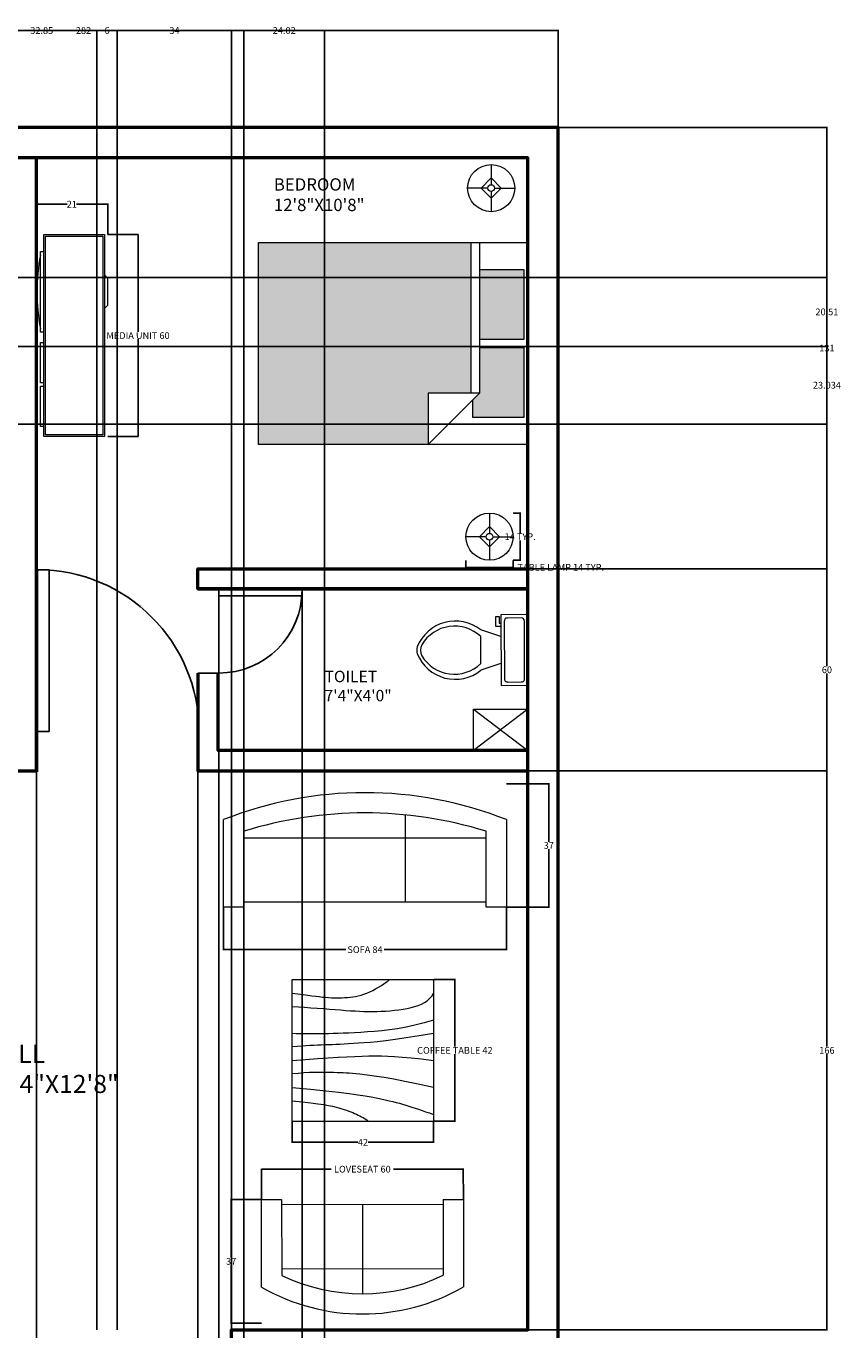
# Model space of a CAD drawing. Units: inches. Extents: x 32 to 429, y 30 to 648.
# Tile 3 of 3: x 187 to 429, y 261 to 648. Entities that reach past the tile are written whole.
import ezdxf

# ---------------------------------------------------------------- set-up
doc = ezdxf.new("R2010")
doc.units = ezdxf.units.IN
doc.header["$MEASUREMENT"] = 0
for name, color, linetype, lineweight in [('A-ANNO-DIMS', 2, 'Continuous', 18), ('A-AREA-IDEN', 7, 'Continuous', 25), ('A-DOOR', 4, 'Continuous', 25), ('A-FLOR-FIXT', 9, 'Continuous', 20), ('A-FURN', 9, 'Continuous', 18), ('A-FURN-PATT', 252, 'Continuous', 13), ('A-WALL', 7, 'Continuous', 50)]:
    doc.layers.add(name, color=color, linetype=linetype, lineweight=lineweight)
doc.styles.get("Standard").update_dxf_attribs({"font": 'arial.ttf'})
doc.dimstyles.get("Standard").update_dxf_attribs({"dimtxt": 2, "dimasz": 0.18, "dimexe": 0.18, "dimexo": 0.0625, "dimgap": 0.09, "dimtad": 0, "dimtih": 1, "dimtoh": 1, "dimrnd": 2, "dimzin": 0, "dimdsep": 46, "dimlunit": 3, "dimtxsty": 'Standard', "dimcen": 0.09, "dimadec": 0, "dimazin": 0, "dimtfac": 1, "dimtofl": 0, "dimtmove": 0, "dimatfit": 3, "dimfxl": 1, "dimtolj": 1, "dimtzin": 0, "dimarcsym": 0})

# ---------------------------------------------------------------- blocks, each defined once
blk = doc.blocks.new('*U3')
for p, q in [((9.5, -6), (9.5, -2)), ((-10, -8.5), (-8, -8.5)), ((-10, -9.5), (-10, -8.5)), ((-7, -9.5), (-10, -9.5)), ((-8, -8.5), (-8, -8)), ((-7, -8), (-7, -9.5)), ((-4, -8), (-6, -14)), ((4, -8), (6, -14)), ((4, -14), (-4, -14))]:
    blk.add_line(p, q)
blk.add_lwpolyline([(10.5, -8), (10.5, 0), (-10.5, 0), (-10.5, -8)], close=True)
for points in [[(-9.5, -2), (-9.5, -6)], [(8.5, -1), (-8.5, -1)], [(-8.5, -7), (8.5, -7)]]:
    blk.add_lwpolyline(points)
for centre, radius, start, end in [((-8.62, -1.88), 0.884, 81.8699, 188.1301), ((8.62, -1.88), 0.884, 351.8699, 98.1301), ((-8.62, -6.12), 0.884, 171.8699, 278.1301), ((8.62, -6.12), 0.884, 261.8699, 8.1301), ((3.52, -21.58), 12.17, 141.4691, 247.9714), ((4.2, -21.82), 11.33, 136.3677, 238.9468), ((-3.52, -21.58), 12.17, 292.0284, 38.5307), ((-4.2, -21.82), 11.33, 301.053, 43.6321), ((0, -27.88), 4, 245.7318, 294.2682), ((0, -29), 4, 254.8605, 285.1395)]:
    blk.add_arc(centre, radius, start, end)
blk = doc.blocks.new('*U6')
for p, q in [((-24, 0), (-24, 6)), ((0, 0), (0, 6))]:
    blk.add_line(p, q)
blk.add_lwpolyline([(0, 0), (0, -24), (-1.75, -24), (-1.75, 0)], close=True)
blk.add_arc((0, 0), 24, 180, 270)
blk = doc.blocks.new('*U8')
for p, q in [((-24, 0), (-24, 6)), ((0, 0), (0, 6))]:
    blk.add_line(p, q)
blk.add_lwpolyline([(0, 0), (0, -24), (-1.75, -24), (-1.75, 0)], close=True)
blk.add_arc((0, 0), 24, 180, 270)
blk = doc.blocks.new('Bed - Queen')
for p, q in [((0, -80.00003), (0, 0)), ((0, 0), (59.99999, 0)), ((59.99999, 0), (59.99999, -80.00003)), ((7.99999, -1.2), (28.79998, -1.2)), ((7.99999, -14.4), (7.99999, -1.2)), ((28.79998, -1.2), (28.79998, -14.4)), ((31.19999, -1.2), (51.99999, -1.2)), ((31.19999, -14.4), (31.19999, -1.2)), ((51.99999, -1.2), (51.99999, -16.4)), ((0, -14.4), (44.8, -14.4)), ((59.99999, -29.6), (44.8, -14.4)), ((44.8, -14.4), (44.8, -29.6)), ((44.8, -16.8), (0, -16.8)), ((51.99999, -16.4), (46.79936, -16.4)), ((44.8, -29.6), (59.99999, -29.6)), ((59.99999, -80.00003), (0, -80.00003))]:
    blk.add_line(p, q)
blk = doc.blocks.new('Entertainment Center')
for p, q in [((-4, 0), (-5, -1)), ((4, 0), (-4, 0)), ((5, -1), (4, 0)), ((-17, -19), (-17, -1)), ((-17, -1), (43, -1)), ((-16.5, -18.5), (-16.5, -1.5)), ((-16.5, -1.5), (42.5, -1.5)), ((42.5, -1.5), (42.5, -18.5)), ((43, -1), (43, -19)), ((43, -19), (-17, -19)), ((42.5, -18.5), (-16.5, -18.5)), ((-12, -20), (-12, -19)), ((12, -19), (12, -20)), ((15, -20), (15, -19)), ((27, -19), (27, -20)), ((28, -20), (28, -19)), ((40, -19), (40, -20)), ((12, -20), (-12, -20)), ((27, -20), (15, -20)), ((40, -20), (28, -20))]:
    blk.add_line(p, q)
blk.add_arc((0, 40), 61, 259.6111, 280.3889)
blk = doc.blocks.new('Lamp - Table')
for p, q in [((0, 7), (0, 1)), ((-1, 0), (-7, 0)), ((0, 3), (-3, 0)), ((-3, 0), (0, -3)), ((3, 0), (0, 3)), ((0, -3), (3, 0)), ((1, 0), (7, 0)), ((0, -1), (0, -7))]:
    blk.add_line(p, q)
for radius in [7, 1]:
    blk.add_circle((0, 0), radius)
blk = doc.blocks.new('Sofa - Roundback 7 ft.')
for p, q in [((-12.00002, -32.4421), (-12.00003, -6.5971)), ((11.99997, -32.4421), (11.99998, -6.5971)), ((-36.000027, -34), (-36.000027, -11.4696)), ((35.99998, -34), (35.99998, -11.4696)), ((-35.999844, -13.3819), (35.9998, -13.3819)), ((-36.000027, -32.4421), (35.99998, -32.4421))]:
    blk.add_line(p, q)
for points in [[(-36.000027, -34), (-42.000027, -34), (-42.000027, -8)], [(41.99998, -8), (41.99998, -34), (35.99998, -34)]]:
    blk.add_lwpolyline(points)
for centre, radius, start, end in [((0, -114.25), 114.25, 68.43141, 111.5686), ((-0.00001, -127.1968), 121.1968, 72.72033, 107.2797)]:
    blk.add_arc(centre, radius, start, end)
blk = doc.blocks.new('Sofa - Roundback Loveseat 5 ft.')
for p, q in [((0, -32.44198), (0, -5.99998)), ((-24, -33.99998), (-24, -11.46958)), ((24.00004, -33.99998), (24.00004, -11.46958)), ((-23.9998, -13.38178), (23.99986, -13.38178)), ((-24, -32.44198), (24.00004, -32.44198))]:
    blk.add_line(p, q)
for points in [[(-24, -33.99998), (-30, -33.99998), (-30, -7.99998)], [(30.00004, -7.99998), (30.00004, -33.99998), (24.00004, -33.99998)]]:
    blk.add_lwpolyline(points)
for centre, radius, start, end in [((0, -60.24998), 60.24998, 60.13715, 119.8628), ((0, -61.38438), 55.38444, 64.32083, 115.6792)]:
    blk.add_arc(centre, radius, start, end)
blk = doc.blocks.new('Table - Square Woodgrain 42 x 42 in.')
blk.add_line((0, -42), (42, -42))
for points in [[(0, -4), (1.704, -4.2172), (3.2358, -4.4188), (4.615, -4.604), (5.8615, -4.7721), (6.9951, -4.9224), (8.0357, -5.0541), (9.0031, -5.1667), (9.9171, -5.2594), (10.7951, -5.3316), (11.6445, -5.3836), (12.4702, -5.4157), (13.277, -5.4283), (14.0698, -5.4217), (14.8535, -5.3964), (15.6331, -5.3526), (16.4133, -5.2908), (17.1986, -5.2103), (17.9913, -5.1062), (18.793, -4.9727), (19.6056, -4.8038), (20.4307, -4.5937), (21.2701, -4.3365), (22.1256, -4.0262), (22.9989, -3.6571), (23.888, -3.2272), (24.7756, -2.7516), (25.6408, -2.2491), (26.4624, -1.7387), (27.2195, -1.2395), (27.891, -0.7703), (28.456, -0.3501), (28.8934, 0.002)], [(0, -42), (0, 0), (42, 0), (42, -42)], [(0, -8), (1.8203, -8.1001), (3.6741, -8.2149), (5.5411, -8.3408), (7.4011, -8.4741), (9.2339, -8.6112), (11.0193, -8.7484), (12.7371, -8.8821), (14.3671, -9.0086), (15.8954, -9.1246), (17.3337, -9.2278), (18.6997, -9.3159), (20.0116, -9.387), (21.2871, -9.4389), (22.5442, -9.4696), (23.8008, -9.477), (25.0749, -9.459), (26.3791, -9.4137), (27.7049, -9.3403), (29.0383, -9.2382), (30.3655, -9.1068), (31.6728, -8.9455), (32.9461, -8.7535), (34.1717, -8.5304), (35.3358, -8.2756), (36.4268, -7.9863), (37.443, -7.6521), (38.3849, -7.2603), (39.253, -6.7986), (40.048, -6.2542), (40.7705, -5.6147), (41.421, -4.8674), (42, -4)], [(42, -12), (39.1784, -12.8621), (36.4519, -13.5654), (33.8246, -14.1294), (31.3004, -14.5731), (28.8832, -14.9161), (26.577, -15.1775), (24.3858, -15.3768), (22.3136, -15.5332), (20.3622, -15.6632), (18.5254, -15.7718), (16.7947, -15.8612), (15.1618, -15.9338), (13.6183, -15.9916), (12.1558, -16.0369), (10.7659, -16.0718), (9.4403, -16.0987), (8.1703, -16.1191), (6.9461, -16.1325), (5.7577, -16.1377), (4.595, -16.1335), (3.4479, -16.1188), (2.3064, -16.0924), (1.1604, -16.0532), (0, -16)], [(42, -16), (37.6529, -16.7365), (33.8802, -17.329), (30.6179, -17.7961), (27.8015, -18.1561), (25.3668, -18.4275), (23.2497, -18.6288), (21.3859, -18.7785), (19.7111, -18.8949), (18.1693, -18.9939), (16.7375, -19.0795), (15.401, -19.1534), (14.1449, -19.217), (12.9544, -19.2717), (11.8148, -19.3191), (10.7113, -19.3606), (9.6291, -19.3976), (8.5534, -19.4323), (7.47, -19.4689), (6.3643, -19.5122), (5.222, -19.5672), (4.0288, -19.6386), (2.7703, -19.7313), (1.4321, -19.8501), (0, -20)], [(0, -24), (3.9243, -23.6805), (7.4766, -23.4138), (10.6891, -23.1954), (13.5943, -23.0205), (16.2247, -22.8847), (18.6125, -22.7832), (20.7903, -22.7116), (22.7903, -22.6651), (24.6563, -22.642), (26.4764, -22.6507), (28.35, -22.7024), (30.3766, -22.8084), (32.6555, -22.98), (35.2861, -23.2283), (38.3678, -23.5645), (42, -24)], [(42, -32), (37.392, -31.017), (33.4585, -30.2231), (30.1291, -29.5949), (27.3334, -29.109), (25.0009, -28.742), (23.0612, -28.4707), (21.4439, -28.2716), (20.0786, -28.1215), (18.8998, -28.0002), (17.8609, -27.9014), (16.9206, -27.8219), (16.0371, -27.7588), (15.1691, -27.709), (14.2748, -27.6693), (13.3128, -27.6368), (12.2415, -27.6083), (11.0295, -27.5824), (9.6867, -27.5643), (8.233, -27.5608), (6.6884, -27.5787), (5.0728, -27.6248), (3.4062, -27.7058), (1.7086, -27.8286), (0, -28)], [(0, -32), (5.4026, -32.5358), (9.9494, -33.019), (13.7424, -33.4553), (16.8834, -33.8505), (19.4743, -34.2106), (21.6171, -34.5413), (23.4136, -34.8486), (24.9657, -35.1382), (26.3614, -35.4156), (27.6332, -35.6841), (28.7995, -35.9467), (29.8788, -36.2064), (30.8897, -36.4661), (31.8507, -36.7288), (32.7802, -36.9973), (33.6968, -37.2747), (34.6175, -37.5635), (35.5531, -37.8651), (36.5128, -38.1805), (37.506, -38.5108), (38.5421, -38.8568), (39.6302, -39.2197), (40.7797, -39.6004), (42, -40)], [(0, -36), (3.0098, -36.2857), (5.5354, -36.5643), (7.6368, -36.8359), (9.374, -37.1009), (10.807, -37.3597), (11.9957, -37.6126), (13.0002, -37.8599), (13.8804, -38.102), (14.6874, -38.3393), (15.4365, -38.5729), (16.1338, -38.8041), (16.7858, -39.0341), (17.3987, -39.264), (17.9787, -39.4952), (18.5322, -39.7288), (19.0655, -39.9662), (19.5832, -40.2081), (20.0842, -40.4544), (20.5657, -40.7046), (21.0249, -40.9581), (21.459, -41.2144), (21.8653, -41.4731), (22.2409, -41.7335), (22.5831, -41.9951)]]:
    blk.add_lwpolyline(points)
blk = doc.blocks.new('*D19')
at = {"layer": 'A-ANNO-DIMS', "color": 0, "lineweight": -2, "transparency": 16777216}
for p, q in [((318, 489.44), (318, 487.22)), ((332, 489.44), (332, 487.22)), ((318.18, 487.4), (331.82, 487.4)), ((332, 487.4), (332.18, 487.4))]:
    blk.add_line(p, q, dxfattribs=at)
at = {"layer": 'A-ANNO-DIMS', "color": 0, "transparency": 16777216}
for points in [[(318.18, 487.43), (318.18, 487.37), (318, 487.4)], [(331.82, 487.43), (331.82, 487.37), (332, 487.4)]]:
    blk.add_solid(points, dxfattribs=at)
at = {"layer": 'Defpoints', "color": 0, "transparency": 16777216}
for p in [(318, 489.5), (332, 489.5), (332, 487.4)]:
    blk.add_point(p, dxfattribs=at)
at = {"layer": 'A-ANNO-DIMS', "color": 0, "transparency": 16777216, "insert": (346.17, 487.4), "char_height": 2, "attachment_point": 5}
blk.add_mtext('\\A1;TABLE LAMP 14 TYP.', dxfattribs=at)
blk = doc.blocks.new('*D20')
at = {"layer": 'A-ANNO-DIMS', "color": 0, "lineweight": -2, "transparency": 16777216}
for p, q in [((332.06, 503.5), (334.28, 503.5)), ((334.1, 503.32), (334.1, 497.59)), ((334.1, 489.68), (334.1, 495.41)), ((332.06, 489.5), (334.28, 489.5))]:
    blk.add_line(p, q, dxfattribs=at)
at = {"layer": 'A-ANNO-DIMS', "color": 0, "transparency": 16777216}
for points in [[(334.07, 503.32), (334.13, 503.32), (334.1, 503.5)], [(334.07, 489.68), (334.13, 489.68), (334.1, 489.5)]]:
    blk.add_solid(points, dxfattribs=at)
at = {"layer": 'Defpoints', "color": 0, "transparency": 16777216}
for p in [(332, 503.5), (334.1, 503.5), (332, 489.5)]:
    blk.add_point(p, dxfattribs=at)
at = {"layer": 'A-ANNO-DIMS', "color": 0, "transparency": 16777216, "insert": (334.1, 496.5), "char_height": 2, "attachment_point": 5}
blk.add_mtext('\\A1;14 TYP.', dxfattribs=at)
blk = doc.blocks.new('*D25')
at = {"layer": 'A-ANNO-DIMS', "color": 0, "lineweight": -2, "transparency": 16777216}
for p, q in [((211.65, 586.21), (220.76, 586.21)), ((220.58, 586.03), (220.58, 557.32)), ((220.58, 526.39), (220.58, 555.1)), ((211.65, 526.21), (220.76, 526.21))]:
    blk.add_line(p, q, dxfattribs=at)
at = {"layer": 'A-ANNO-DIMS', "color": 0, "transparency": 16777216}
for points in [[(220.55, 586.03), (220.61, 586.03), (220.58, 586.21)], [(220.55, 526.39), (220.61, 526.39), (220.58, 526.21)]]:
    blk.add_solid(points, dxfattribs=at)
at = {"layer": 'Defpoints', "color": 0, "transparency": 16777216}
for p in [(211.58, 586.21), (211.58, 526.21), (220.58, 526.21)]:
    blk.add_point(p, dxfattribs=at)
at = {"layer": 'A-ANNO-DIMS', "color": 0, "transparency": 16777216, "insert": (220.58, 556.21), "char_height": 2, "attachment_point": 5}
blk.add_mtext('\\A1;MEDIA UNIT 60', dxfattribs=at)
blk = doc.blocks.new('*D26')
at = {"layer": 'A-ANNO-DIMS', "color": 0, "lineweight": -2, "transparency": 16777216}
for p, q in [((190.25, 586.27), (190.25, 595.39)), ((190.43, 595.21), (199.57, 595.21)), ((211.4, 595.21), (202.26, 595.21)), ((211.58, 586.27), (211.58, 595.39))]:
    blk.add_line(p, q, dxfattribs=at)
at = {"layer": 'A-ANNO-DIMS', "color": 0, "transparency": 16777216}
for points in [[(190.43, 595.24), (190.43, 595.18), (190.25, 595.21)], [(211.4, 595.24), (211.4, 595.18), (211.58, 595.21)]]:
    blk.add_solid(points, dxfattribs=at)
at = {"layer": 'Defpoints', "color": 0, "transparency": 16777216}
for p in [(211.58, 595.21), (190.25, 586.21), (211.58, 586.21)]:
    blk.add_point(p, dxfattribs=at)
at = {"layer": 'A-ANNO-DIMS', "color": 0, "transparency": 16777216, "insert": (200.92, 595.21), "char_height": 2, "attachment_point": 5}
blk.add_mtext('\\A1;21', dxfattribs=at)
blk = doc.blocks.new('*D27')
at = {"layer": 'A-ANNO-DIMS', "color": 0, "lineweight": -2, "transparency": 16777216}
for p, q in [((246, 386.44), (246, 373.72)), ((330, 386.44), (330, 373.72)), ((246.18, 373.9), (282.29, 373.9)), ((329.82, 373.9), (293.71, 373.9))]:
    blk.add_line(p, q, dxfattribs=at)
at = {"layer": 'A-ANNO-DIMS', "color": 0, "transparency": 16777216}
for points in [[(246.18, 373.93), (246.18, 373.87), (246, 373.9)], [(329.82, 373.93), (329.82, 373.87), (330, 373.9)]]:
    blk.add_solid(points, dxfattribs=at)
at = {"layer": 'Defpoints', "color": 0, "transparency": 16777216}
for p in [(246, 386.5), (330, 386.5), (330, 373.9)]:
    blk.add_point(p, dxfattribs=at)
at = {"layer": 'A-ANNO-DIMS', "color": 0, "transparency": 16777216, "insert": (288, 373.9), "char_height": 2, "attachment_point": 5}
blk.add_mtext('\\A1;SOFA 84', dxfattribs=at)
blk = doc.blocks.new('*D28')
at = {"layer": 'A-ANNO-DIMS', "color": 0, "lineweight": -2, "transparency": 16777216}
for p, q in [((330.06, 423.17), (342.78, 423.17)), ((342.6, 422.99), (342.6, 405.95)), ((342.6, 386.68), (342.6, 403.72)), ((330.06, 386.5), (342.78, 386.5))]:
    blk.add_line(p, q, dxfattribs=at)
at = {"layer": 'A-ANNO-DIMS', "color": 0, "transparency": 16777216}
for points in [[(342.57, 422.99), (342.63, 422.99), (342.6, 423.17)], [(342.57, 386.68), (342.63, 386.68), (342.6, 386.5)]]:
    blk.add_solid(points, dxfattribs=at)
at = {"layer": 'Defpoints', "color": 0, "transparency": 16777216}
for p in [(330, 423.17), (342.6, 423.17), (330, 386.5)]:
    blk.add_point(p, dxfattribs=at)
at = {"layer": 'A-ANNO-DIMS', "color": 0, "transparency": 16777216, "insert": (342.6, 404.83), "char_height": 2, "attachment_point": 5}
blk.add_mtext('\\A1;37', dxfattribs=at)
blk = doc.blocks.new('*D29')
at = {"layer": 'A-ANNO-DIMS', "color": 0, "lineweight": -2, "transparency": 16777216}
for p, q in [((257.23, 299.74), (257.22, 308.86)), ((257.4, 308.68), (277.98, 308.71)), ((317.04, 308.76), (296.46, 308.74)), ((317.23, 299.83), (317.22, 308.94))]:
    blk.add_line(p, q, dxfattribs=at)
at = {"layer": 'A-ANNO-DIMS', "color": 0, "transparency": 16777216}
for points in [[(257.4, 308.71), (257.4, 308.65), (257.22, 308.68)], [(317.04, 308.79), (317.04, 308.73), (317.22, 308.76)]]:
    blk.add_solid(points, dxfattribs=at)
at = {"layer": 'Defpoints', "color": 0, "transparency": 16777216}
for p in [(257.22, 308.68), (257.23, 299.68), (317.23, 299.76)]:
    blk.add_point(p, dxfattribs=at)
at = {"layer": 'A-ANNO-DIMS', "color": 0, "transparency": 16777216, "insert": (287.22, 308.72), "char_height": 2, "attachment_point": 5}
blk.add_mtext('\\A1;LOVESEAT 60', dxfattribs=at)
blk = doc.blocks.new('*D30')
at = {"layer": 'A-ANNO-DIMS', "color": 0, "lineweight": -2, "transparency": 16777216}
for p, q in [((257.17, 299.68), (248.05, 299.67)), ((248.23, 299.49), (248.26, 282.45)), ((248.28, 263.18), (248.26, 280.22)), ((257.22, 263.01), (248.1, 263))]:
    blk.add_line(p, q, dxfattribs=at)
at = {"layer": 'A-ANNO-DIMS', "color": 0, "transparency": 16777216}
for points in [[(248.26, 299.49), (248.2, 299.49), (248.23, 299.67)], [(248.31, 263.18), (248.25, 263.18), (248.28, 263)]]:
    blk.add_solid(points, dxfattribs=at)
at = {"layer": 'Defpoints', "color": 0, "transparency": 16777216}
for p in [(257.23, 299.68), (248.28, 263), (257.28, 263.01)]:
    blk.add_point(p, dxfattribs=at)
at = {"layer": 'A-ANNO-DIMS', "color": 0, "transparency": 16777216, "insert": (248.26, 281.34), "char_height": 2, "attachment_point": 5}
blk.add_mtext('\\A1;37', dxfattribs=at)
blk = doc.blocks.new('*D31')
at = {"layer": 'A-ANNO-DIMS', "color": 0, "lineweight": -2, "transparency": 16777216}
for p, q in [((308.46, 365), (314.88, 365)), ((314.7, 364.82), (314.7, 345.13)), ((314.7, 323.18), (314.7, 342.88)), ((308.46, 323), (314.88, 323))]:
    blk.add_line(p, q, dxfattribs=at)
at = {"layer": 'A-ANNO-DIMS', "color": 0, "transparency": 16777216}
for points in [[(314.67, 364.82), (314.73, 364.82), (314.7, 365)], [(314.67, 323.18), (314.73, 323.18), (314.7, 323)]]:
    blk.add_solid(points, dxfattribs=at)
at = {"layer": 'Defpoints', "color": 0, "transparency": 16777216}
for p in [(308.4, 365), (314.7, 365), (308.4, 323)]:
    blk.add_point(p, dxfattribs=at)
at = {"layer": 'A-ANNO-DIMS', "color": 0, "transparency": 16777216, "insert": (314.7, 344), "char_height": 2, "attachment_point": 5}
blk.add_mtext('\\A1;COFFEE TABLE 42', dxfattribs=at)
blk = doc.blocks.new('*D32')
at = {"layer": 'A-ANNO-DIMS', "color": 0, "lineweight": -2, "transparency": 16777216}
for p, q in [((266.4, 322.94), (266.4, 316.52)), ((308.4, 322.94), (308.4, 316.52)), ((266.58, 316.7), (285.85, 316.7)), ((308.22, 316.7), (288.95, 316.7))]:
    blk.add_line(p, q, dxfattribs=at)
at = {"layer": 'A-ANNO-DIMS', "color": 0, "transparency": 16777216}
for points in [[(266.58, 316.73), (266.58, 316.67), (266.4, 316.7)], [(308.22, 316.73), (308.22, 316.67), (308.4, 316.7)]]:
    blk.add_solid(points, dxfattribs=at)
at = {"layer": 'Defpoints', "color": 0, "transparency": 16777216}
for p in [(266.4, 323), (308.4, 323), (308.4, 316.7)]:
    blk.add_point(p, dxfattribs=at)
at = {"layer": 'A-ANNO-DIMS', "color": 0, "transparency": 16777216, "insert": (287.4, 316.7), "char_height": 2, "attachment_point": 5}
blk.add_mtext('\\A1;42', dxfattribs=at)
blk = doc.blocks.new('*D33')
at = {"layer": 'A-ANNO-DIMS', "color": 0, "lineweight": -2, "transparency": 16777216}
for p, q in [((63.39, 618.06), (63.39, 646.97)), ((63.57, 646.79), (202.09, 646.79)), ((345.21, 646.79), (206.7, 646.79)), ((345.39, 618.06), (345.39, 646.97))]:
    blk.add_line(p, q, dxfattribs=at)
at = {"layer": 'A-ANNO-DIMS', "color": 0, "transparency": 16777216}
for points in [[(63.57, 646.82), (63.57, 646.76), (63.39, 646.79)], [(345.21, 646.82), (345.21, 646.76), (345.39, 646.79)]]:
    blk.add_solid(points, dxfattribs=at)
at = {"layer": 'Defpoints', "color": 0, "transparency": 16777216}
for p in [(345.39, 646.79), (63.39, 617.99), (345.39, 617.99)]:
    blk.add_point(p, dxfattribs=at)
at = {"layer": 'A-ANNO-DIMS', "color": 0, "transparency": 16777216, "insert": (204.39, 646.79), "char_height": 2, "attachment_point": 5}
blk.add_mtext('\\A1;282', dxfattribs=at)
blk = doc.blocks.new('*D40')
at = {"layer": 'A-ANNO-DIMS', "color": 0, "lineweight": -2, "transparency": 16777216}
for p, q in [((336.46, 426.99), (425.41, 426.99)), ((425.23, 426.81), (425.23, 345.1)), ((425.23, 261.17), (425.23, 342.88)), ((336.46, 260.99), (425.41, 260.99))]:
    blk.add_line(p, q, dxfattribs=at)
at = {"layer": 'A-ANNO-DIMS', "color": 0, "transparency": 16777216}
for points in [[(425.2, 426.81), (425.26, 426.81), (425.23, 426.99)], [(425.2, 261.17), (425.26, 261.17), (425.23, 260.99)]]:
    blk.add_solid(points, dxfattribs=at)
at = {"layer": 'Defpoints', "color": 0, "transparency": 16777216}
for p in [(336.39, 426.99), (425.23, 426.99), (336.39, 260.99)]:
    blk.add_point(p, dxfattribs=at)
at = {"layer": 'A-ANNO-DIMS', "color": 0, "transparency": 16777216, "insert": (425.23, 343.99), "char_height": 2, "attachment_point": 5}
blk.add_mtext('\\A1;166', dxfattribs=at)
blk = doc.blocks.new('*D41')
at = {"layer": 'A-ANNO-DIMS', "color": 0, "lineweight": -2, "transparency": 16777216}
for p, q in [((336.46, 486.99), (425.41, 486.99)), ((425.23, 486.81), (425.23, 458.1)), ((425.23, 427.17), (425.23, 455.88)), ((336.46, 426.99), (425.41, 426.99))]:
    blk.add_line(p, q, dxfattribs=at)
at = {"layer": 'A-ANNO-DIMS', "color": 0, "transparency": 16777216}
for points in [[(425.2, 486.81), (425.26, 486.81), (425.23, 486.99)], [(425.2, 427.17), (425.26, 427.17), (425.23, 426.99)]]:
    blk.add_solid(points, dxfattribs=at)
at = {"layer": 'Defpoints', "color": 0, "transparency": 16777216}
for p in [(336.39, 486.99), (425.23, 486.99), (336.39, 426.99)]:
    blk.add_point(p, dxfattribs=at)
at = {"layer": 'A-ANNO-DIMS', "color": 0, "transparency": 16777216, "insert": (425.23, 456.99), "char_height": 2, "attachment_point": 5}
blk.add_mtext('\\A1;60', dxfattribs=at)
blk = doc.blocks.new('*D42')
at = {"layer": 'A-ANNO-DIMS', "color": 0, "lineweight": -2, "transparency": 16777216}
for p, q in [((345.46, 617.99), (425.41, 617.99)), ((425.23, 617.81), (425.23, 553.6)), ((425.23, 487.17), (425.23, 551.38)), ((336.46, 486.99), (425.41, 486.99))]:
    blk.add_line(p, q, dxfattribs=at)
at = {"layer": 'A-ANNO-DIMS', "color": 0, "transparency": 16777216}
for points in [[(425.2, 617.81), (425.26, 617.81), (425.23, 617.99)], [(425.2, 487.17), (425.26, 487.17), (425.23, 486.99)]]:
    blk.add_solid(points, dxfattribs=at)
at = {"layer": 'Defpoints', "color": 0, "transparency": 16777216}
for p in [(345.39, 617.99), (425.23, 617.99), (336.39, 486.99)]:
    blk.add_point(p, dxfattribs=at)
at = {"layer": 'A-ANNO-DIMS', "color": 0, "transparency": 16777216, "insert": (425.23, 552.49), "char_height": 2, "attachment_point": 5}
blk.add_mtext('\\A1;131', dxfattribs=at)
blk = doc.blocks.new('*D45')
at = {"layer": 'A-ANNO-DIMS', "color": 0, "lineweight": -2, "transparency": 16777216}
for p, q in [((190.39, 426.93), (190.39, 31.01)), ((238.39, 426.93), (238.39, 31.01)), ((190.57, 31.19), (212.83, 31.19)), ((238.21, 31.19), (215.96, 31.19))]:
    blk.add_line(p, q, dxfattribs=at)
at = {"layer": 'A-ANNO-DIMS', "color": 0, "transparency": 16777216}
for points in [[(190.57, 31.22), (190.57, 31.16), (190.39, 31.19)], [(238.21, 31.22), (238.21, 31.16), (238.39, 31.19)]]:
    blk.add_solid(points, dxfattribs=at)
at = {"layer": 'Defpoints', "color": 0, "transparency": 16777216}
for p in [(190.39, 426.99), (238.39, 426.99), (238.39, 31.19)]:
    blk.add_point(p, dxfattribs=at)
at = {"layer": 'A-ANNO-DIMS', "color": 0, "transparency": 16777216, "insert": (214.39, 31.19), "char_height": 2, "attachment_point": 5}
blk.add_mtext('\\A1;48', dxfattribs=at)
blk = doc.blocks.new('*D46')
at = {"layer": 'A-ANNO-DIMS', "color": 0, "lineweight": -2, "transparency": 16777216}
for p, q in [((175.55, 261.06), (175.55, 646.97)), ((175.73, 646.79), (188.5, 646.79)), ((208.21, 646.79), (195.44, 646.79)), ((208.39, 261.06), (208.39, 646.97))]:
    blk.add_line(p, q, dxfattribs=at)
at = {"layer": 'A-ANNO-DIMS', "color": 0, "transparency": 16777216}
for points in [[(175.73, 646.82), (175.73, 646.76), (175.55, 646.79)], [(208.21, 646.82), (208.21, 646.76), (208.39, 646.79)]]:
    blk.add_solid(points, dxfattribs=at)
at = {"layer": 'Defpoints', "color": 0, "transparency": 16777216}
for p in [(208.39, 646.79), (175.55, 260.99), (208.39, 260.99)]:
    blk.add_point(p, dxfattribs=at)
at = {"layer": 'A-ANNO-DIMS', "color": 0, "transparency": 16777216, "insert": (191.97, 646.79), "char_height": 2, "attachment_point": 5}
blk.add_mtext('\\A1;32.85', dxfattribs=at)
blk = doc.blocks.new('*D47')
at = {"layer": 'A-ANNO-DIMS', "color": 0, "lineweight": -2, "transparency": 16777216}
for p, q in [((214.39, 261.06), (214.39, 646.97)), ((214.57, 646.79), (229.88, 646.79)), ((248.21, 646.79), (232.91, 646.79)), ((248.39, 261.06), (248.39, 646.97))]:
    blk.add_line(p, q, dxfattribs=at)
at = {"layer": 'A-ANNO-DIMS', "color": 0, "transparency": 16777216}
for points in [[(214.57, 646.82), (214.57, 646.76), (214.39, 646.79)], [(248.21, 646.82), (248.21, 646.76), (248.39, 646.79)]]:
    blk.add_solid(points, dxfattribs=at)
at = {"layer": 'Defpoints', "color": 0, "transparency": 16777216}
for p in [(248.39, 646.79), (214.39, 260.99), (248.39, 260.99)]:
    blk.add_point(p, dxfattribs=at)
at = {"layer": 'A-ANNO-DIMS', "color": 0, "transparency": 16777216, "insert": (231.39, 646.79), "char_height": 2, "attachment_point": 5}
blk.add_mtext('\\A1;34', dxfattribs=at)
blk = doc.blocks.new('*D48')
at = {"layer": 'A-ANNO-DIMS', "color": 0, "lineweight": -2, "transparency": 16777216}
for p, q in [((208.39, 261.06), (208.39, 646.97)), ((208.57, 646.79), (210.64, 646.79)), ((214.21, 646.79), (212.14, 646.79)), ((214.39, 261.06), (214.39, 646.97))]:
    blk.add_line(p, q, dxfattribs=at)
at = {"layer": 'A-ANNO-DIMS', "color": 0, "transparency": 16777216}
for points in [[(208.57, 646.82), (208.57, 646.76), (208.39, 646.79)], [(214.21, 646.82), (214.21, 646.76), (214.39, 646.79)]]:
    blk.add_solid(points, dxfattribs=at)
at = {"layer": 'Defpoints', "color": 0, "transparency": 16777216}
for p in [(214.39, 646.79), (208.39, 260.99), (214.39, 260.99)]:
    blk.add_point(p, dxfattribs=at)
at = {"layer": 'A-ANNO-DIMS', "color": 0, "transparency": 16777216, "insert": (211.39, 646.79), "char_height": 2, "attachment_point": 5}
blk.add_mtext('\\A1;6', dxfattribs=at)
blk = doc.blocks.new('*D50')
at = {"layer": 'A-ANNO-DIMS', "color": 0, "lineweight": -2, "transparency": 16777216}
for p, q in [((147.08, 552.99), (425.41, 552.99)), ((425.23, 552.81), (425.23, 542.59)), ((425.23, 530.14), (425.23, 540.36)), ((147.08, 529.96), (425.41, 529.96))]:
    blk.add_line(p, q, dxfattribs=at)
at = {"layer": 'A-ANNO-DIMS', "color": 0, "transparency": 16777216}
for points in [[(425.2, 552.81), (425.26, 552.81), (425.23, 552.99)], [(425.2, 530.14), (425.26, 530.14), (425.23, 529.96)]]:
    blk.add_solid(points, dxfattribs=at)
at = {"layer": 'Defpoints', "color": 0, "transparency": 16777216}
for p in [(147.02, 552.99), (147.02, 529.96), (425.23, 529.96)]:
    blk.add_point(p, dxfattribs=at)
at = {"layer": 'A-ANNO-DIMS', "color": 0, "transparency": 16777216, "insert": (425.23, 541.48), "char_height": 2, "attachment_point": 5}
blk.add_mtext('\\A1;23.034', dxfattribs=at)
blk = doc.blocks.new('*D51')
at = {"layer": 'A-ANNO-DIMS', "color": 0, "lineweight": -2, "transparency": 16777216}
for p, q in [((244.58, 478.88), (244.58, 31.01)), ((269.32, 478.88), (269.32, 31.01)), ((244.76, 31.19), (253.47, 31.19)), ((269.14, 31.19), (260.43, 31.19))]:
    blk.add_line(p, q, dxfattribs=at)
at = {"layer": 'A-ANNO-DIMS', "color": 0, "transparency": 16777216}
for points in [[(244.76, 31.22), (244.76, 31.16), (244.58, 31.19)], [(269.14, 31.22), (269.14, 31.16), (269.32, 31.19)]]:
    blk.add_solid(points, dxfattribs=at)
at = {"layer": 'Defpoints', "color": 0, "transparency": 16777216}
for p in [(244.58, 478.95), (269.32, 478.95), (269.32, 31.19)]:
    blk.add_point(p, dxfattribs=at)
at = {"layer": 'A-ANNO-DIMS', "color": 0, "transparency": 16777216, "insert": (256.95, 31.19), "char_height": 2, "attachment_point": 5}
blk.add_mtext('\\A1;24.74', dxfattribs=at)
blk = doc.blocks.new('*D52')
at = {"layer": 'A-ANNO-DIMS', "color": 0, "lineweight": -2, "transparency": 16777216}
for p, q in [((252, 232.11), (252, 646.97)), ((252.18, 646.79), (260.54, 646.79)), ((275.84, 646.79), (267.48, 646.79)), ((276.02, 232.11), (276.02, 646.97))]:
    blk.add_line(p, q, dxfattribs=at)
at = {"layer": 'A-ANNO-DIMS', "color": 0, "transparency": 16777216}
for points in [[(252.18, 646.82), (252.18, 646.76), (252, 646.79)], [(275.84, 646.82), (275.84, 646.76), (276.02, 646.79)]]:
    blk.add_solid(points, dxfattribs=at)
at = {"layer": 'Defpoints', "color": 0, "transparency": 16777216}
for p in [(276.02, 646.79), (252, 232.04), (276.02, 232.04)]:
    blk.add_point(p, dxfattribs=at)
at = {"layer": 'A-ANNO-DIMS', "color": 0, "transparency": 16777216, "insert": (264.01, 646.79), "char_height": 2, "attachment_point": 5}
blk.add_mtext('\\A1;24.02', dxfattribs=at)
blk = doc.blocks.new('*D56')
at = {"layer": 'A-ANNO-DIMS', "color": 0, "lineweight": -2, "transparency": 16777216}
for p, q in [((72.46, 573.5), (425.41, 573.5)), ((425.23, 573.32), (425.23, 564.36)), ((425.23, 553.17), (425.23, 562.14)), ((72.46, 552.99), (425.41, 552.99))]:
    blk.add_line(p, q, dxfattribs=at)
at = {"layer": 'A-ANNO-DIMS', "color": 0, "transparency": 16777216}
for points in [[(425.2, 573.32), (425.26, 573.32), (425.23, 573.5)], [(425.2, 553.17), (425.26, 553.17), (425.23, 552.99)]]:
    blk.add_solid(points, dxfattribs=at)
at = {"layer": 'Defpoints', "color": 0, "transparency": 16777216}
for p in [(72.39, 573.5), (425.23, 573.5), (72.39, 552.99)]:
    blk.add_point(p, dxfattribs=at)
at = {"layer": 'A-ANNO-DIMS', "color": 0, "transparency": 16777216, "insert": (425.23, 563.25), "char_height": 2, "attachment_point": 5}
blk.add_mtext('\\A1;20.51', dxfattribs=at)

msp = doc.modelspace()

# ---------------------------------------------------------------- hatches: boundary and pattern name
at = {"layer": 'A-FURN-PATT'}
h = msp.add_hatch(dxfattribs=at)
h.set_pattern_fill('DOTS', color=256)
h.paths.add_polyline_path([(335.194, 575.8763), (321.994, 575.8763), (321.994, 555.0763), (335.194, 555.0763)])
h.paths.add_polyline_path([(335.194, 552.6763), (321.994, 552.6763), (321.994, 539.0763), (319.994, 537.0763), (319.994, 531.8763), (335.194, 531.8763)])
h.paths.add_polyline_path([(319.594, 583.8763), (256.3939, 583.8763), (256.3939, 523.8763), (306.794, 523.8763), (306.794, 539.0763), (319.594, 539.0763)])
h = msp.add_hatch(dxfattribs=at)
h.set_pattern_fill('DOTS', color=256)
h.paths.add_polyline_path([(319.594, 583.8763), (256.3939, 583.8763), (256.3939, 523.8763), (306.794, 523.8763), (306.794, 539.0763), (319.594, 539.0763)])

# ---------------------------------------------------------------- linework, layer by layer
at = {"layer": 'A-FLOR-FIXT'}
for p, q in [((320.2761, 445.3289), (336.3942, 432.9929)), ((336.3942, 445.3289), (320.2761, 432.9929))]:
    msp.add_line(p, q, dxfattribs=at)
msp.add_lwpolyline([(336.3942, 432.9929), (320.2761, 432.9929), (320.2761, 445.3289), (336.3942, 445.3289)], close=True, dxfattribs=at)
at = {"layer": 'A-WALL'}
for points in [[(208.3942, 59.9929), (345.3942, 59.9929), (345.3942, 617.9929), (63.3942, 617.9929), (63.3942, 59.9929)], [(248.394, 254.9928), (248.394, 260.9928), (336.394, 260.9928), (336.394, 608.9928), (72.394, 608.9928), (72.394, 59.9928)], [(336.3942, 608.9929), (184.3942, 608.9929), (184.3942, 432.9929), (184.3942, 426.9929), (190.3942, 426.9929), (190.3942, 608.9929)], [(244.3942, 480.9929), (336.3942, 480.9929), (238.3942, 480.9929), (238.3942, 486.9929), (336.3942, 486.9929)], [(238.3942, 456.0096), (238.3942, 426.9929), (336.3942, 426.9929)], [(336.3942, 432.9929), (244.3942, 432.9929), (244.3942, 456.0073)]]:
    msp.add_lwpolyline(points, dxfattribs=at)

# ---------------------------------------------------------------- block references
at = {"layer": 'A-DOOR'}
for name, p, xscale, yscale, zscale, rotation in [('*U8', (190.681, 438.7075), 2.000008218349355, 2.000008218349355, 2.000008218349355, 180), ('*U6', (244.5793, 480.7509), 1.030886389251549, 1.030886389251549, 1.030886389251549, 90.00000000000003)]:
    msp.add_blockref(name, p, dxfattribs=dict(at, xscale=xscale, yscale=yscale, zscale=zscale, rotation=rotation))
at = {"layer": 'A-FLOR-FIXT', "rotation": 270.1882894233738}
msp.add_blockref('*U3', (336.3942, 462.8786), dxfattribs=at)
at = {"layer": 'A-FURN'}
for name, p in [('Lamp - Table', (325.5, 600)), ('Lamp - Table', (325, 496.5)), ('Sofa - Roundback 7 ft.', (288, 420.5)), ('Table - Square Woodgrain 42 x 42 in.', (266.3997, 364.9999))]:
    msp.add_blockref(name, p, dxfattribs=at)
for name, p, rotation in [('Entertainment Center', (211.5826, 569.2085), 270), ('Bed - Queen', (336.394, 583.8763), 270), ('Sofa - Roundback Loveseat 5 ft.', (287.2787, 265.7227), 180.0784294782872)]:
    msp.add_blockref(name, p, dxfattribs=dict(at, rotation=rotation))

# ---------------------------------------------------------------- texts
at = {"layer": 'A-AREA-IDEN', "attachment_point": 1}
for s, width, gutter_width, insert, char_height in [('BEDROOM\\P12\'8"X10\'8"', 18.261984, 18.262, (260.925, 602.912), 3.652397), ('TOILET\\P7\'4"X4\'0"', 8.502953, 17.0059, (275.997, 456.7021), 3.40118), ('HALL\\P21\'4"X12\'8"', 49.260324, 26.8336, (175.2397, 345.6521), 5.366729)]:
    msp.add_mtext_dynamic_manual_height_columns(s, width=width, gutter_width=gutter_width, heights=[0], dxfattribs=dict(at, insert=insert, char_height=char_height))

# ---------------------------------------------------------------- dimensions: what is measured, and where the dimension line sits
at = {"layer": 'A-ANNO-DIMS'}
for base, p1, p2, override, picture, middle in [((345.3942, 646.7929), (63.3942, 617.9929), (345.3942, 617.9929), {"dimdec": 0, "dimlfac": 1, "dimrnd": 0, "dimzin": 0, "dimdsep": 46, "dimlunit": 2}, '*D33', (204.3942, 646.7929)), ((208.3942, 646.7929), (175.5464, 260.9929), (208.3942, 260.9929), {"dimdec": 2, "dimlfac": 1, "dimrnd": 0, "dimzin": 0, "dimdsep": 46, "dimlunit": 2}, '*D46', (191.9703, 646.7929)), ((214.3942, 646.7929), (208.3942, 260.9929), (214.3942, 260.9929), {"dimdec": 0, "dimlfac": 1, "dimrnd": 0, "dimzin": 0, "dimdsep": 46, "dimlunit": 2}, '*D48', (211.3942, 646.7929)), ((248.394, 646.7929), (214.3942, 260.9929), (248.394, 260.9928), {"dimdec": 0, "dimlfac": 1, "dimrnd": 0, "dimzin": 0, "dimdsep": 46, "dimlunit": 2}, '*D47', (231.3941, 646.7929)), ((276.0156, 646.7929), (251.997, 232.0437), (276.0156, 232.0437), {"dimdec": 2, "dimlfac": 1, "dimrnd": 0, "dimzin": 0, "dimdsep": 46, "dimlunit": 2}, '*D52', (264.0063, 646.7929)), ((211.5826, 595.2085), (190.2493, 586.2085), (211.5826, 586.2085), {"dimdec": 0, "dimlfac": 1, "dimrnd": 0, "dimzin": 0, "dimdsep": 46, "dimlunit": 2}, '*D26', (200.9159, 595.2085)), ((269.3206, 31.1928), (244.5793, 478.9469), (269.3206, 478.9469), {"dimdec": 2, "dimlfac": 1, "dimrnd": 0, "dimzin": 0, "dimdsep": 46, "dimlunit": 2}, '*D51', (256.95, 31.1928)), ((238.3942, 31.1928), (190.3942, 426.9929), (238.3942, 426.9929), {"dimdec": 0, "dimlfac": 1, "dimrnd": 0, "dimzin": 0, "dimdsep": 46, "dimlunit": 2}, '*D45', (214.3942, 31.1928)), ((308.3997, 316.6996), (266.3997, 322.9999), (308.3997, 322.9999), {"dimdec": 0, "dimlfac": 1, "dimrnd": 0, "dimzin": 0, "dimdsep": 46, "dimlunit": 2}, '*D32', (287.3997, 316.6996))]:
    dim = msp.add_linear_dim(base=base, p1=p1, p2=p2, dimstyle='Standard', override=override, dxfattribs=at)
    dim.commit()
    dim.dimension.update_dxf_attribs({"geometry": picture, "text_midpoint": middle})
for base, p1, p2, angle, override, picture, middle in [((425.2284, 617.9929), (336.3942, 486.9929), (345.3942, 617.9929), 90, {"dimdec": 0, "dimlfac": 1, "dimrnd": 0, "dimzin": 0, "dimdsep": 46, "dimlunit": 2}, '*D42', (425.2284, 552.4929)), ((425.2284, 573.5041), (72.3942, 552.9929), (72.3942, 573.5041), 90, {"dimdec": 2, "dimlfac": 1, "dimrnd": 0, "dimzin": 0, "dimdsep": 46, "dimlunit": 2}, '*D56', (425.2284, 563.2485)), ((425.22842, 529.95843), (147.01917, 552.99291), (147.01917, 529.95843), 90, {"dimdec": 3, "dimlfac": 1, "dimrnd": 0, "dimzin": 0, "dimdsep": 46, "dimlunit": 2}, '*D50', (425.22842, 541.47567)), ((425.2284, 486.9929), (336.3942, 426.9929), (336.3942, 486.9929), 90, {"dimdec": 0, "dimlfac": 1, "dimrnd": 0, "dimzin": 0, "dimdsep": 46, "dimlunit": 2}, '*D41', (425.2284, 456.9929)), ((425.2284, 426.9929), (336.394, 260.9928), (336.3942, 426.9929), 90, {"dimdec": 0, "dimlfac": 1, "dimrnd": 0, "dimzin": 0, "dimdsep": 46, "dimlunit": 2}, '*D40', (425.2284, 343.9929)), ((342.6, 423.1667), (330, 386.5), (330, 423.1667), 90, {"dimdec": 0, "dimlfac": 1, "dimrnd": 0, "dimzin": 0, "dimdsep": 46, "dimlunit": 2}, '*D28', (342.6, 404.8333)), ((248.2824, 263.0026), (257.2322, 299.6815), (257.2823, 263.0149), 270.078429, {"dimdec": 0, "dimlfac": 1, "dimrnd": 0, "dimzin": 0, "dimdsep": 46, "dimlunit": 2}, '*D30', (248.2573, 281.3359))]:
    dim = msp.add_linear_dim(base=base, p1=p1, p2=p2, angle=angle, dimstyle='Standard', override=override, dxfattribs=at)
    dim.commit()
    dim.dimension.update_dxf_attribs({"geometry": picture, "text_midpoint": middle})
for base, p1, p2, angle, text, picture, middle in [((220.5826, 526.2085), (211.5826, 586.2085), (211.5826, 526.2085), 270, 'MEDIA UNIT <>', '*D25', (220.5826, 556.2085)), ((334.1, 503.5), (332, 489.5), (332, 503.5), 90, '<> TYP.', '*D20', (334.1, 496.5)), ((314.7, 365.0019), (308.3997, 322.9999), (308.3997, 365.0019), 90, 'COFFEE TABLE <>', '*D31', (314.7, 344.0009)), ((257.2198, 308.6815), (317.2321, 299.7637), (257.2322, 299.6815), 180.078429, 'LOVESEAT <>', '*D29', (287.2198, 308.7226))]:
    dim = msp.add_linear_dim(base=base, p1=p1, p2=p2, angle=angle, text=text, dimstyle='Standard', override={"dimdec": 0, "dimlfac": 1, "dimrnd": 0, "dimzin": 0, "dimdsep": 46, "dimlunit": 2}, dxfattribs=at)
    dim.commit()
    dim.dimension.update_dxf_attribs({"geometry": picture, "text_midpoint": middle})
for base, p1, p2, text, picture, middle in [((332, 487.4), (318, 489.5), (332, 489.5), 'TABLE LAMP <> TYP.', '*D19', (346.169, 487.4)), ((330, 373.9), (246, 386.5), (330, 386.5), 'SOFA <>', '*D27', (288, 373.9))]:
    dim = msp.add_linear_dim(base=base, p1=p1, p2=p2, text=text, dimstyle='Standard', override={"dimdec": 0, "dimlfac": 1, "dimrnd": 0, "dimzin": 0, "dimdsep": 46, "dimlunit": 2}, dxfattribs=at)
    dim.commit()
    dim.dimension.update_dxf_attribs({"geometry": picture, "text_midpoint": middle})

doc.saveas('drawing.dxf')
